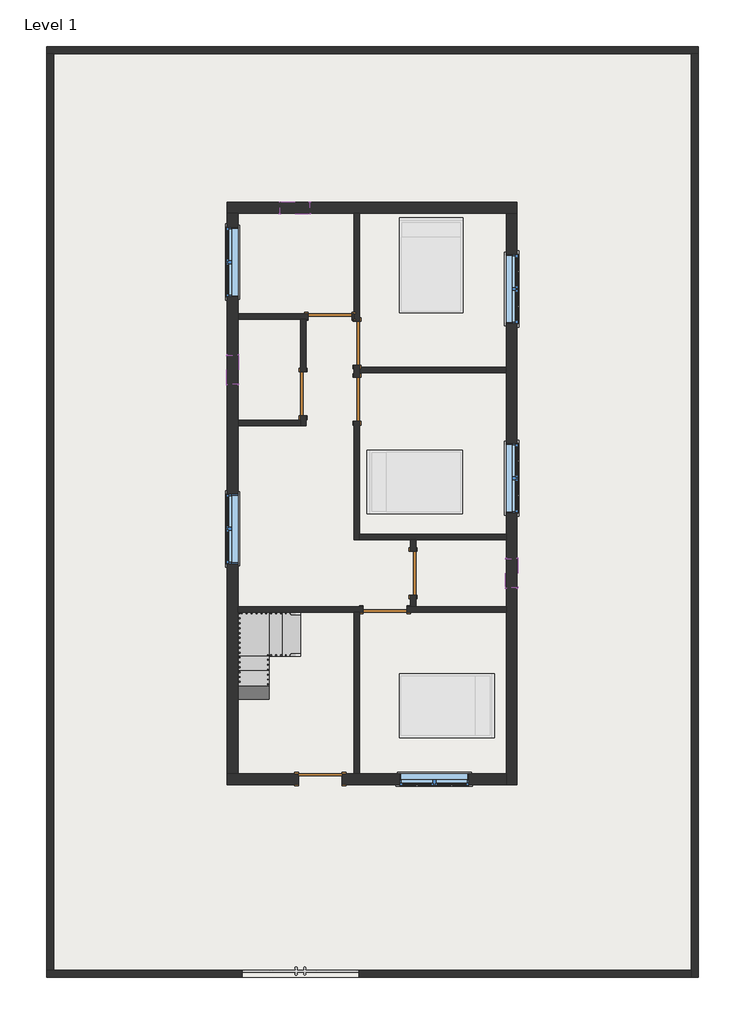
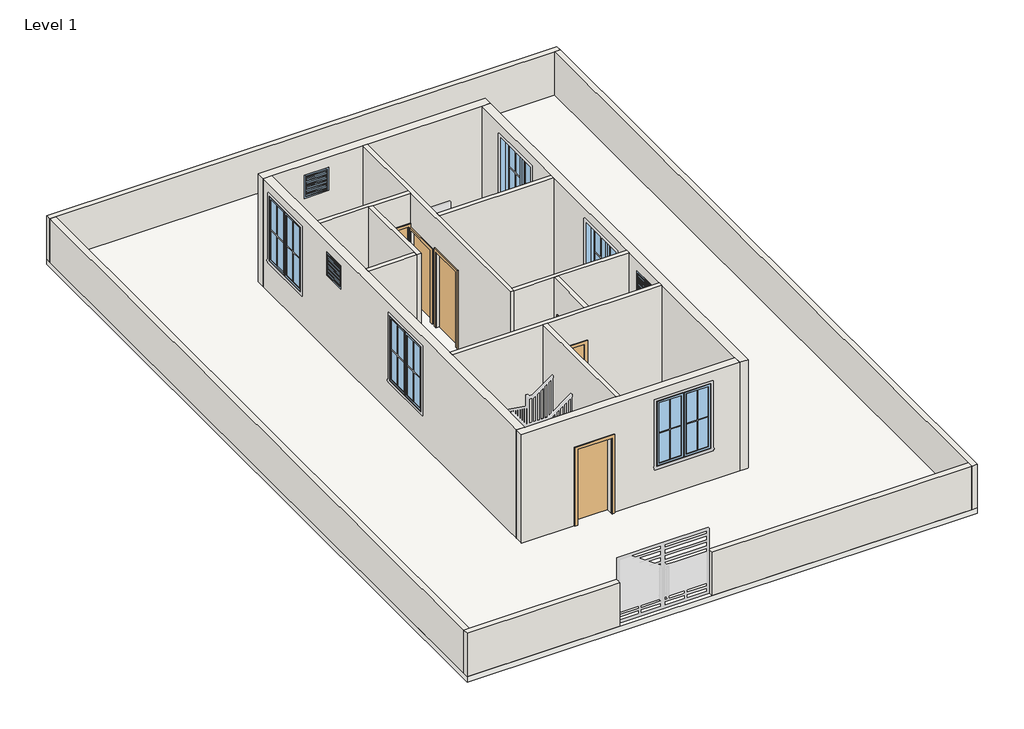
# One storey, part 1 of 2: 18 walls, 8 windows, 7 doors, 1 slab, 1 stair flight.
"""IFC4 building model written with IfcOpenShell, lengths in millimetres."""

from ifc_helpers import new_model, si_unit, frame, origin, origin_with_axes, place, context, project, spatial, polyline, outline, extrude, faceted_brep, transform, mapped, element, save
from components import door_5e62189b, door_17d80c48, door_e5f9f3c4, door_305aa2a5, door_0ca8825f, window_9ac97e1a, window_f2d8fef0

model = new_model("IFC4")

# Units and contexts
model_context = context("Model", 3, world=origin())
ifc_project = project(units=[si_unit("LENGTHUNIT", "METRE", prefix="MILLI")], contexts=[model_context])

# Site, building, storey
site = spatial("IfcSite", under=ifc_project)
building = spatial("IfcBuilding", under=site)
storey = spatial("IfcBuildingStorey", under=building, Name="Level 1", Elevation=0.0)

# Doors
placement = place(None, origin())
door_shape = door_5e62189b(model_context)
element("IfcDoor", 1, ObjectType="Single-Flush : 36\" x 80\"", at=placement, inside=storey, context=model_context, shape_type="MappedRepresentation", body=[
    mapped(door_shape, transform((-2690.3389285, 2204.6069249, 0.0), x_axis=(0.0, -1.0, 0.0), y_axis=(1.0, 0.0, 0.0), z_axis=(0.0, 0.0, 1.0))),
])
element("IfcDoor", 2, ObjectType="Single-Flush : 36\" x 80\"", at=placement, inside=storey, context=model_context, shape_type="MappedRepresentation", body=[
    mapped(door_shape, transform((-404.3389285, -1522.8430751, 0.0), x_axis=(0.0, 1.0, 0.0), y_axis=(-1.0, 0.0, 0.0), z_axis=(0.0, 0.0, 1.0))),
])
door_2_shape = door_17d80c48(model_context)
element("IfcDoor", 3, ObjectType="Single-Flush : 36\" x 80\"", at=placement, inside=storey, context=model_context, shape_type="MappedRepresentation", body=[
    mapped(door_2_shape, transform((-1572.7389285, 3258.7069249, 0.0), x_axis=(0.0, -1.0, 0.0), y_axis=(1.0, 0.0, 0.0), z_axis=(0.0, 0.0, 1.0))),
])
door_3_shape = door_e5f9f3c4(model_context)
element("IfcDoor", 4, ObjectType="Single-Flush : 36\" x 84\"", at=placement, inside=storey, context=model_context, shape_type="MappedRepresentation", body=[
    mapped(door_3_shape, transform((-2131.5389285, 3817.5069249, 0.0), x_axis=(1.0, 0.0, 0.0), y_axis=(0.0, 1.0, 0.0), z_axis=(0.0, 0.0, 1.0))),
])
element("IfcDoor", 5, ObjectType="Single-Flush : 36\" x 84\"", at=placement, inside=storey, context=model_context, shape_type="MappedRepresentation", body=[
    mapped(door_3_shape, transform((-988.5389285, -2278.4930751, 0.0), x_axis=(-1.0, 0.0, 0.0), y_axis=(0.0, -1.0, 0.0), z_axis=(0.0, 0.0, 1.0))),
])
door_4_shape = door_305aa2a5(model_context)
element("IfcDoor", 6, ObjectType="Single-Flush : 36\" x 84\"", at=placement, inside=storey, context=model_context, shape_type="MappedRepresentation", body=[
    mapped(door_4_shape, transform((-1572.7389285, 2090.3069249, 0.0), x_axis=(0.0, 1.0, 0.0), y_axis=(-1.0, 0.0, 0.0), z_axis=(0.0, 0.0, 1.0))),
])
door_5_shape = door_0ca8825f(model_context)
element("IfcDoor", 7, ObjectType="Single-Flush : 36\" x 84\"", at=placement, inside=storey, context=model_context, shape_type="MappedRepresentation", body=[
    mapped(door_5_shape, transform((-2334.7389285, -5802.7430751, 0.0), x_axis=(1.0, 0.0, 0.0), y_axis=(0.0, 1.0, 0.0), z_axis=(0.0, 0.0, 1.0))),
])

# Slab
element("IfcSlab", 8, ObjectType="FLOOR 6\"", at=placement, inside=storey, context=model_context, shape_type="SweptSolid", body=[
    extrude(outline(polyline([(5532.8162989, 9427.0671147), (5532.8162989, -9927.7328853), (-8030.7837011, -9927.7328853), (-8030.7837011, 9427.0671147), (5532.8162989, 9427.0671147)])), frame((0.0, 0.0, -152.4), z_axis=(0.0, 0.0, 1.0), x_axis=(1.0, 0.0, 0.0)), (0.0, 0.0, 1.0), 152.4),
])

# Stair flight
element("IfcStairFlight", 9, ObjectType="3/4\" Nosing", at=placement, inside=storey, context=model_context, shape_type="Brep", body=[
    faceted_brep([(-2747.4889285, -3250.0430751, 217.7142857), (-2747.4889285, -2335.6430751, 217.7142857), (-3128.4889285, -2335.6430751, 217.7142857), (-3128.4889285, -3250.0430751, 217.7142857), (-3128.4889285, -3250.0430751, 154.2142857), (-2753.0451785, -3250.0430751, 154.2142857), (-2753.0451785, -2335.6430751, 154.2142857), (-3128.4889285, -2335.6430751, 154.2142857)], [[[0, 1, 2, 3]], [[0, 3, 4, 5]], [[2, 1, 6, 7]], [[1, 0, 5, 6]], [[4, 7, 6, 5]], [[7, 4, 3, 2]]]),
    faceted_brep([(-3128.4889285, -3250.0430751, 435.4285714), (-3128.4889285, -2335.6430751, 435.4285714), (-3401.5389285, -2335.6430751, 435.4285714), (-3401.5389285, -3250.0430751, 435.4285714), (-3401.5389285, -3250.0430751, 371.9285714), (-3134.0451785, -3250.0430751, 371.9285714), (-3134.0451785, -2335.6430751, 371.9285714), (-3401.5389285, -2335.6430751, 371.9285714)], [[[0, 1, 2, 3]], [[0, 3, 4, 5]], [[2, 1, 6, 7]], [[1, 0, 5, 6]], [[4, 7, 6, 5]], [[7, 4, 3, 2]]]),
    faceted_brep([(-3401.5389285, -3269.0930751, 653.1428571), (-3401.5389285, -3250.0430751, 653.1428571), (-3401.5389285, -2335.6430751, 653.1428571), (-4042.8889285, -2335.6430751, 653.1428571), (-4042.8889285, -3269.0930751, 653.1428571), (-3401.5389285, -3269.0930751, 589.6428571), (-3401.5389285, -3250.0430751, 589.6428571), (-3407.0951785, -3250.0430751, 589.6428571), (-3407.0951785, -2335.6430751, 589.6428571), (-4042.8889285, -2335.6430751, 589.6428571), (-4042.8889285, -3269.0930751, 589.6428571), (-3401.5389285, -3250.0430751, 870.8571429), (-4042.8889285, -3250.0430751, 870.8571429), (-4042.8889285, -3289.4456691, 870.8571429), (-4042.8889285, -3573.8930751, 870.8571429), (-3401.5389285, -3573.8930751, 870.8571429), (-3401.5389285, -3289.4456691, 870.8571429), (-3401.5389285, -3573.8930751, 792.8571605), (-3401.5389285, -3289.4456691, 589.6428571), (-4042.8889285, -3289.4456691, 589.6428571), (-4042.8889285, -3573.8930751, 792.8571605), (-3401.5389285, -3554.8430751, 1088.5714286), (-4042.8889285, -3554.8430751, 1088.5714286), (-4042.8889285, -3878.6930751, 1088.5714286), (-3401.5389285, -3878.6930751, 1088.5714286), (-3401.5389285, -3878.6930751, 1010.6117202), (-4042.8889285, -3878.6930751, 1010.6117202), (-3401.5389285, -3859.6430751, 1306.2857143), (-4042.8889285, -3859.6430751, 1306.2857143), (-4042.8889285, -4183.4930751, 1306.2857143), (-3401.5389285, -4183.4930751, 1306.2857143), (-3401.5389285, -4183.4930751, 1228.36628), (-4042.8889285, -4183.4930751, 1228.36628), (-3401.5389285, -4164.4430751, 1524.0), (-4042.8889285, -4164.4430751, 1524.0), (-4042.8889285, -4488.2930751, 1524.0), (-3401.5389285, -4488.2930751, 1524.0), (-3401.5389285, -4488.2930751, 1446.1208397), (-4042.8889285, -4488.2930751, 1446.1208397), (-3401.5389285, -4792.8112092, 1741.7142857), (-3401.5389285, -4469.2430751, 1741.7142857), (-4042.8889285, -4469.2430751, 1741.7142857), (-4042.8889285, -4792.8112092, 1741.7142857), (-3401.5389285, -4773.7612092, 1959.4285714), (-3401.5389285, -5117.90743, 1959.4285714), (-3401.5389285, -5117.90743, 1895.9285714), (-4042.8889285, -4792.8112092, 1663.6740294), (-4042.8889285, -4773.7612092, 1959.4285714), (-4042.8889285, -5117.90743, 1959.4285714), (-4042.8889285, -5688.4430751, 1959.4285714), (-3401.5389285, -5688.4430751, 1959.4285714), (-4042.8889285, -5117.90743, 1895.9285714), (-4042.8889285, -5688.4430751, 1895.9285714), (-3401.5389285, -5688.4430751, 1895.9285714)], [[[0, 1, 2, 3, 4]], [[1, 0, 5, 6]], [[7, 1, 6]], [[3, 2, 8, 9]], [[4, 3, 9, 10]], [[11, 12, 13, 14, 15, 16]], [[0, 11, 16, 15, 17, 18, 5]], [[12, 4, 10, 19, 20, 14, 13]], [[21, 22, 23, 24]], [[21, 24, 25, 17, 15]], [[23, 22, 14, 20, 26]], [[27, 28, 29, 30]], [[27, 30, 31, 25, 24]], [[29, 28, 23, 26, 32]], [[33, 34, 35, 36]], [[33, 36, 37, 31, 30]], [[35, 34, 29, 32, 38]], [[39, 40, 41, 42]], [[39, 43, 44, 45, 37, 36, 40]], [[42, 41, 35, 38, 46]], [[43, 47, 48, 49, 50, 44]], [[47, 42, 46, 51, 52, 49, 48]], [[50, 49, 52, 53]], [[2, 1, 7, 8]], [[0, 4, 12, 11]], [[15, 14, 22, 21]], [[24, 23, 28, 27]], [[30, 29, 34, 33]], [[36, 35, 41, 40]], [[39, 42, 47, 43]], [[18, 19, 10, 9, 8, 7, 6, 5]], [[19, 18, 17, 25, 31, 37, 45, 51, 46, 38, 32, 26, 20]], [[45, 53, 52, 51]], [[53, 45, 44, 50]]]),
    faceted_brep([(-3401.5389285, -4773.7612092, 2177.1428571), (-3401.5389285, -5688.4430751, 2177.1428571), (-3128.4889285, -5688.4430751, 2177.1428571), (-3128.4889285, -4773.7612092, 2177.1428571), (-3395.9826785, -4773.7612092, 2113.6428571), (-3128.4889285, -4773.7612092, 2113.6428571), (-3395.9826785, -5688.4430751, 2113.6428571), (-3128.4889285, -5688.4430751, 2113.6428571)], [[[0, 1, 2, 3]], [[4, 0, 3, 5]], [[2, 1, 6, 7]], [[1, 0, 4, 6]], [[5, 7, 6, 4]], [[7, 5, 3, 2]]]),
    faceted_brep([(-3128.4889285, -4773.7612092, 2394.8571429), (-3128.4889285, -5688.4430751, 2394.8571429), (-2793.6303845, -5688.4430751, 2394.8571429), (-2793.6303845, -4773.7612092, 2394.8571429), (-2793.6303845, -4773.7612092, 2331.3571429), (-3122.9326785, -4773.7612092, 2331.3571429), (-3122.9326785, -5688.4430751, 2331.3571429), (-2793.6303845, -5688.4430751, 2331.3571429)], [[[0, 1, 2, 3]], [[0, 3, 4, 5]], [[2, 1, 6, 7]], [[3, 2, 7, 4]], [[1, 0, 5, 6]], [[6, 5, 4, 7]]]),
])

# Walls
element("IfcWall", 10, ObjectType="CMD 6\"", at=placement, inside=storey, context=model_context, shape_type="Brep", body=[
    faceted_brep([(-8030.7837011, 9274.6671147, 0.0), (-7878.3837011, 9274.6671147, 0.0), (5380.4162989, 9274.6671147, 0.0), (5532.8162989, 9274.6671147, 0.0), (5532.8162989, 9274.6671147, 1219.2), (5380.4162989, 9274.6671147, 1219.2), (-7878.3837011, 9274.6671147, 1219.2), (-8030.7837011, 9274.6671147, 1219.2), (-8030.7837011, 9427.0671147, 0.0), (-8030.7837011, 9427.0671147, 1219.2), (5532.8162989, 9427.0671147, 1219.2), (5532.8162989, 9427.0671147, 0.0)], [[[0, 1, 2, 3, 4, 5, 6, 7]], [[8, 9, 10, 11]], [[3, 2, 1, 0, 8, 11]], [[7, 6, 5, 4, 10, 9]], [[4, 3, 11, 10]], [[0, 7, 9, 8]]]),
])
element("IfcWall", 11, ObjectType="CMD 6\"", at=placement, inside=storey, context=model_context, shape_type="Brep", body=[
    faceted_brep([(5380.4162989, 9274.6671147, 0.0), (5380.4162989, -9775.3328853, 0.0), (5380.4162989, -9927.7328853, 0.0), (5380.4162989, -9927.7328853, 1219.2), (5380.4162989, -9775.3328853, 1219.2), (5380.4162989, 9274.6671147, 1219.2), (5532.8162989, 9274.6671147, 0.0), (5532.8162989, 9274.6671147, 1219.2), (5532.8162989, -9927.7328853, 1219.2), (5532.8162989, -9927.7328853, 0.0)], [[[0, 1, 2, 3, 4, 5]], [[6, 7, 8, 9]], [[2, 1, 0, 6, 9]], [[5, 4, 3, 8, 7]], [[0, 5, 7, 6]], [[3, 2, 9, 8]]]),
])
element("IfcWall", 12, ObjectType="CMD 6\"", at=placement, inside=storey, context=model_context, shape_type="SweptSolid", body=[
    extrude(outline(polyline([(-1528.2889285, -9775.3328853), (5380.4162989, -9775.3328853), (5380.4162989, -9927.7328853), (-1528.2889285, -9927.7328853), (-1528.2889285, -9775.3328853)])), origin_with_axes(), (0.0, 0.0, 1.0), 1219.2),
])
element("IfcWall", 13, ObjectType="CMD 6\"", at=placement, inside=storey, context=model_context, shape_type="SweptSolid", body=[
    extrude(outline(polyline([(-7878.3837011, 9274.6671147), (-7878.3837011, -9775.3328853), (-8030.7837011, -9775.3328853), (-8030.7837011, 9274.6671147), (-7878.3837011, 9274.6671147)])), origin_with_axes(), (0.0, 0.0, 1.0), 1219.2),
])
element("IfcWall", 14, ObjectType="CMD 6\"", at=placement, inside=storey, context=model_context, shape_type="Brep", body=[
    faceted_brep([(-3966.6889285, -9775.3328853, 0.0), (-7878.3837011, -9775.3328853, 0.0), (-8030.7837011, -9775.3328853, 0.0), (-8030.7837011, -9775.3328853, 1219.2), (-7878.3837011, -9775.3328853, 1219.2), (-3966.6889285, -9775.3328853, 1219.2), (-3966.6889285, -9927.7328853, 0.0), (-3966.6889285, -9927.7328853, 1219.2), (-8030.7837011, -9927.7328853, 1219.2), (-8030.7837011, -9927.7328853, 0.0)], [[[0, 1, 2, 3, 4, 5]], [[6, 7, 8, 9]], [[2, 1, 0, 6, 9]], [[5, 4, 3, 8, 7]], [[0, 5, 7, 6]], [[3, 2, 9, 8]]]),
])
element("IfcWall", 15, ObjectType="WALL 4.5\"", at=placement, inside=storey, context=model_context, shape_type="Brep", body=[
    faceted_brep([(-1629.8889285, 2801.5069249, 2032.0), (-1629.8889285, 2801.5069249, 0.0), (-1629.8889285, 2547.5069249, 0.0), (-1629.8889285, 2547.5069249, 2133.6), (-1629.8889285, 1633.1069249, 2133.6), (-1629.8889285, 1633.1069249, 0.0), (-1629.8889285, -824.3430751, 0.0), (-1629.8889285, -824.3430751, 3048.0), (-1629.8889285, 3760.3569249, 3048.0), (-1629.8889285, 3874.6569249, 3048.0), (-1629.8889285, 5957.4569249, 3048.0), (-1629.8889285, 5957.4569249, 0.0), (-1629.8889285, 3874.6569249, 0.0), (-1629.8889285, 3760.3569249, 0.0), (-1629.8889285, 3715.9069249, 0.0), (-1629.8889285, 3715.9069249, 2032.0), (-1515.5889285, 2547.5069249, 0.0), (-1515.5889285, 2642.7569249, 0.0), (-1515.5889285, 2757.0569249, 0.0), (-1515.5889285, 2801.5069249, 0.0), (-1515.5889285, 2801.5069249, 2032.0), (-1515.5889285, 3715.9069249, 2032.0), (-1515.5889285, 3715.9069249, 0.0), (-1515.5889285, 5957.4569249, 0.0), (-1515.5889285, 5957.4569249, 3048.0), (-1515.5889285, 2757.0569249, 3048.0), (-1515.5889285, 2642.7569249, 3048.0), (-1515.5889285, -710.0430751, 3048.0), (-1515.5889285, -824.3430751, 3048.0), (-1515.5889285, -824.3430751, 0.0), (-1515.5889285, -710.0430751, 0.0), (-1515.5889285, 1633.1069249, 0.0), (-1515.5889285, 1633.1069249, 2133.6), (-1515.5889285, 2547.5069249, 2133.6)], [[[0, 1, 2, 3, 4, 5, 6, 7, 8, 9, 10, 11, 12, 13, 14, 15]], [[16, 17, 18, 19, 20, 21, 22, 23, 24, 25, 26, 27, 28, 29, 30, 31, 32, 33]], [[31, 30, 29, 6, 5]], [[2, 1, 19, 18, 17, 16]], [[14, 13, 12, 11, 23, 22]], [[7, 6, 29, 28]], [[11, 10, 24, 23]], [[3, 2, 16, 33]], [[4, 3, 33, 32]], [[5, 4, 32, 31]], [[20, 19, 1, 0]], [[21, 20, 0, 15]], [[22, 21, 15, 14]], [[10, 9, 8, 7, 28, 27, 26, 25, 24]]]),
])
element("IfcWall", 16, ObjectType="WALL 4.5\"", at=placement, inside=storey, context=model_context, shape_type="Brep", body=[
    faceted_brep([(1532.4110715, -710.0430751, 0.0), (-1515.5889285, -710.0430751, 0.0), (-1515.5889285, -710.0430751, 3048.0), (1532.4110715, -710.0430751, 3048.0), (1532.4110715, -824.3430751, 0.0), (1532.4110715, -824.3430751, 3048.0), (-347.1889285, -824.3430751, 3048.0), (-461.4889285, -824.3430751, 3048.0), (-1515.5889285, -824.3430751, 3048.0), (-1515.5889285, -824.3430751, 0.0), (-461.4889285, -824.3430751, 0.0), (-347.1889285, -824.3430751, 0.0)], [[[0, 1, 2, 3]], [[4, 5, 6, 7, 8, 9, 10, 11]], [[1, 0, 4, 11, 10, 9]], [[0, 3, 5, 4]], [[2, 1, 9, 8]], [[3, 2, 8, 7, 6, 5]]]),
])
element("IfcWall", 17, ObjectType="WALL 4.5\"", at=placement, inside=storey, context=model_context, shape_type="SweptSolid", body=[
    extrude(outline(polyline([(-1515.5889285, 2757.0569249), (1532.4110715, 2757.0569249), (1532.4110715, 2642.7569249), (-1515.5889285, 2642.7569249), (-1515.5889285, 2757.0569249)])), origin_with_axes(), (0.0, 0.0, 1.0), 3048.0),
])
element("IfcWall", 18, ObjectType="WALL 4.5\"", at=placement, inside=storey, context=model_context, shape_type="Brep", body=[
    faceted_brep([(-1674.3389285, 3760.3569249, 2133.6), (-1674.3389285, 3760.3569249, 0.0), (-1629.8889285, 3760.3569249, 0.0), (-1629.8889285, 3760.3569249, 3048.0), (-2633.1889285, 3760.3569249, 3048.0), (-2747.4889285, 3760.3569249, 3048.0), (-4042.8889285, 3760.3569249, 3048.0), (-4042.8889285, 3760.3569249, 0.0), (-2747.4889285, 3760.3569249, 0.0), (-2633.1889285, 3760.3569249, 0.0), (-2588.7389285, 3760.3569249, 0.0), (-2588.7389285, 3760.3569249, 2133.6), (-1629.8889285, 3874.6569249, 0.0), (-1674.3389285, 3874.6569249, 0.0), (-1674.3389285, 3874.6569249, 2133.6), (-2588.7389285, 3874.6569249, 2133.6), (-2588.7389285, 3874.6569249, 0.0), (-4042.8889285, 3874.6569249, 0.0), (-4042.8889285, 3874.6569249, 3048.0), (-1629.8889285, 3874.6569249, 3048.0)], [[[0, 1, 2, 3, 4, 5, 6, 7, 8, 9, 10, 11]], [[12, 13, 14, 15, 16, 17, 18, 19]], [[2, 1, 13, 12]], [[10, 9, 8, 7, 17, 16]], [[7, 6, 18, 17]], [[3, 2, 12, 19]], [[14, 13, 1, 0]], [[15, 14, 0, 11]], [[16, 15, 11, 10]], [[6, 5, 4, 3, 19, 18]]]),
])
element("IfcWall", 19, ObjectType="WALL 4.5\"", at=placement, inside=storey, context=model_context, shape_type="Brep", body=[
    faceted_brep([(-2747.4889285, 1747.4069249, 2032.0), (-2747.4889285, 1747.4069249, 0.0), (-2747.4889285, 1652.1569249, 0.0), (-2747.4889285, 1537.8569249, 0.0), (-2747.4889285, 1537.8569249, 3048.0), (-2747.4889285, 1652.1569249, 3048.0), (-2747.4889285, 3760.3569249, 3048.0), (-2747.4889285, 3760.3569249, 0.0), (-2747.4889285, 2661.8069249, 0.0), (-2747.4889285, 2661.8069249, 2032.0), (-2633.1889285, 1537.8569249, 0.0), (-2633.1889285, 1747.4069249, 0.0), (-2633.1889285, 1747.4069249, 2032.0), (-2633.1889285, 2661.8069249, 2032.0), (-2633.1889285, 2661.8069249, 0.0), (-2633.1889285, 3760.3569249, 0.0), (-2633.1889285, 3760.3569249, 3048.0), (-2633.1889285, 1537.8569249, 3048.0)], [[[0, 1, 2, 3, 4, 5, 6, 7, 8, 9]], [[10, 11, 12, 13, 14, 15, 16, 17]], [[8, 7, 15, 14]], [[3, 2, 1, 11, 10]], [[7, 6, 16, 15]], [[4, 3, 10, 17]], [[12, 11, 1, 0]], [[13, 12, 0, 9]], [[14, 13, 9, 8]], [[6, 5, 4, 17, 16]]]),
])
element("IfcWall", 20, ObjectType="WALL 4.5\"", at=placement, inside=storey, context=model_context, shape_type="SweptSolid", body=[
    extrude(outline(polyline([(-4042.8889285, 1652.1569249), (-2747.4889285, 1652.1569249), (-2747.4889285, 1537.8569249), (-4042.8889285, 1537.8569249), (-4042.8889285, 1652.1569249)])), origin_with_axes(), (0.0, 0.0, 1.0), 3048.0),
])
element("IfcWall", 21, ObjectType="WALL 4.5\"", at=placement, inside=storey, context=model_context, shape_type="Brep", body=[
    faceted_brep([(-4042.8889285, -2335.6430751, 0.0), (-1629.8889285, -2335.6430751, 0.0), (-1515.5889285, -2335.6430751, 0.0), (-1445.7389285, -2335.6430751, 0.0), (-1445.7389285, -2335.6430751, 2133.6), (-531.3389285, -2335.6430751, 2133.6), (-531.3389285, -2335.6430751, 0.0), (1532.4110715, -2335.6430751, 0.0), (1532.4110715, -2335.6430751, 3048.0), (-1515.5889285, -2335.6430751, 3048.0), (-1629.8889285, -2335.6430751, 3048.0), (-4042.8889285, -2335.6430751, 3048.0), (-1445.7389285, -2221.3430751, 2133.6), (-1445.7389285, -2221.3430751, 0.0), (-4042.8889285, -2221.3430751, 0.0), (-4042.8889285, -2221.3430751, 3048.0), (-461.4889285, -2221.3430751, 3048.0), (-347.1889285, -2221.3430751, 3048.0), (1532.4110715, -2221.3430751, 3048.0), (1532.4110715, -2221.3430751, 0.0), (-347.1889285, -2221.3430751, 0.0), (-461.4889285, -2221.3430751, 0.0), (-531.3389285, -2221.3430751, 0.0), (-531.3389285, -2221.3430751, 2133.6)], [[[0, 1, 2, 3, 4, 5, 6, 7, 8, 9, 10, 11]], [[12, 13, 14, 15, 16, 17, 18, 19, 20, 21, 22, 23]], [[14, 13, 3, 2, 1, 0]], [[22, 21, 20, 19, 7, 6]], [[8, 7, 19, 18]], [[0, 11, 15, 14]], [[4, 3, 13, 12]], [[5, 4, 12, 23]], [[6, 5, 23, 22]], [[11, 10, 9, 8, 18, 17, 16, 15]]]),
])
element("IfcWall", 22, ObjectType="WALL 4.5\"", at=placement, inside=storey, context=model_context, shape_type="SweptSolid", body=[
    extrude(outline(polyline([(-824.3430751, 0.0), (-1065.6430751, 0.0), (-1065.6430751, 2032.0), (-1980.0430751, 2032.0), (-1980.0430751, 0.0), (-2221.3430751, 0.0), (-2221.3430751, 3048.0), (-824.3430751, 3048.0), (-824.3430751, 0.0)])), frame((-461.4889285, 0.0, 0.0), z_axis=(1.0, 0.0, 0.0), x_axis=(0.0, 1.0, 0.0)), (0.0, 0.0, 1.0), 114.3),
])
element("IfcWall", 23, ObjectType="WALL 4.5\"", at=placement, inside=storey, context=model_context, shape_type="SweptSolid", body=[
    extrude(outline(polyline([(-1629.8889285, -5688.4430751), (-1629.8889285, -2335.6430751), (-1515.5889285, -2335.6430751), (-1515.5889285, -5688.4430751), (-1629.8889285, -5688.4430751)])), origin_with_axes(), (0.0, 0.0, 1.0), 3048.0),
])
element("IfcWall", 24, ObjectType="WALL 9\"", at=placement, inside=storey, context=model_context, shape_type="Brep", body=[
    faceted_brep([(-4271.4889285, 5957.4569249, 0.0), (-4042.8889285, 5957.4569249, 0.0), (-1629.8889285, 5957.4569249, 0.0), (-1515.5889285, 5957.4569249, 0.0), (1532.4110715, 5957.4569249, 0.0), (1761.0110715, 5957.4569249, 0.0), (1761.0110715, 5957.4569249, 3048.0), (1532.4110715, 5957.4569249, 3048.0), (-1515.5889285, 5957.4569249, 3048.0), (-1629.8889285, 5957.4569249, 3048.0), (-4042.8889285, 5957.4569249, 3048.0), (-4271.4889285, 5957.4569249, 3048.0), (-2560.1639285, 5957.4569249, 2743.2), (-2560.1639285, 5957.4569249, 2133.6), (-3169.7639285, 5957.4569249, 2133.6), (-3169.7639285, 5957.4569249, 2743.2), (-4271.4889285, 6186.0569249, 0.0), (-4271.4889285, 6186.0569249, 3048.0), (1761.0110715, 6186.0569249, 3048.0), (1761.0110715, 6186.0569249, 0.0), (-2560.1639285, 6186.0569249, 2743.2), (-3169.7639285, 6186.0569249, 2743.2), (-3169.7639285, 6186.0569249, 2133.6), (-2560.1639285, 6186.0569249, 2133.6)], [[[0, 1, 2, 3, 4, 5, 6, 7, 8, 9, 10, 11], [12, 13, 14, 15]], [[16, 17, 18, 19], [20, 21, 22, 23]], [[5, 4, 3, 2, 1, 0, 16, 19]], [[6, 5, 19, 18]], [[0, 11, 17, 16]], [[13, 12, 20, 23]], [[14, 13, 23, 22]], [[15, 14, 22, 21]], [[12, 15, 21, 20]], [[11, 10, 9, 8, 7, 6, 18, 17]]]),
])
element("IfcWall", 25, ObjectType="WALL 9\"", at=placement, inside=storey, context=model_context, shape_type="Brep", body=[
    faceted_brep([(1532.4110715, 5957.4569249, 0.0), (1532.4110715, 2757.0569249, 0.0), (1532.4110715, 2642.7569249, 0.0), (1532.4110715, -710.0430751, 0.0), (1532.4110715, -824.3430751, 0.0), (1532.4110715, -2221.3430751, 0.0), (1532.4110715, -2335.6430751, 0.0), (1532.4110715, -5688.4430751, 0.0), (1532.4110715, -5917.0430751, 0.0), (1532.4110715, -5917.0430751, 3048.0), (1532.4110715, -5688.4430751, 3048.0), (1532.4110715, -2335.6430751, 3048.0), (1532.4110715, -2221.3430751, 3048.0), (1532.4110715, -824.3430751, 3048.0), (1532.4110715, -710.0430751, 3048.0), (1532.4110715, 2642.7569249, 3048.0), (1532.4110715, 2757.0569249, 3048.0), (1532.4110715, 5957.4569249, 3048.0), (1532.4110715, 3661.9319249, 2743.2), (1532.4110715, 3661.9319249, 914.4), (1532.4110715, 5109.7319249, 914.4), (1532.4110715, 5109.7319249, 2743.2), (1532.4110715, -271.8930751, 2743.2), (1532.4110715, -271.8930751, 914.4), (1532.4110715, 1175.9069249, 914.4), (1532.4110715, 1175.9069249, 2743.2), (1532.4110715, -1827.6430751, 2743.2), (1532.4110715, -1827.6430751, 2133.6), (1532.4110715, -1218.0430751, 2133.6), (1532.4110715, -1218.0430751, 2743.2), (1761.0110715, 5957.4569249, 0.0), (1761.0110715, 5957.4569249, 3048.0), (1761.0110715, -5917.0430751, 3048.0), (1761.0110715, -5917.0430751, 0.0), (1761.0110715, 3661.9319249, 2743.2), (1761.0110715, 5109.7319249, 2743.2), (1761.0110715, 5109.7319249, 914.4), (1761.0110715, 3661.9319249, 914.4), (1761.0110715, -271.8930751, 2743.2), (1761.0110715, 1175.9069249, 2743.2), (1761.0110715, 1175.9069249, 914.4), (1761.0110715, -271.8930751, 914.4), (1761.0110715, -1827.6430751, 2743.2), (1761.0110715, -1218.0430751, 2743.2), (1761.0110715, -1218.0430751, 2133.6), (1761.0110715, -1827.6430751, 2133.6)], [[[0, 1, 2, 3, 4, 5, 6, 7, 8, 9, 10, 11, 12, 13, 14, 15, 16, 17], [18, 19, 20, 21], [22, 23, 24, 25], [26, 27, 28, 29]], [[30, 31, 32, 33], [34, 35, 36, 37], [38, 39, 40, 41], [42, 43, 44, 45]], [[8, 7, 6, 5, 4, 3, 2, 1, 0, 30, 33]], [[0, 17, 31, 30]], [[9, 8, 33, 32]], [[19, 18, 34, 37]], [[20, 19, 37, 36]], [[21, 20, 36, 35]], [[18, 21, 35, 34]], [[23, 22, 38, 41]], [[24, 23, 41, 40]], [[25, 24, 40, 39]], [[22, 25, 39, 38]], [[27, 26, 42, 45]], [[28, 27, 45, 44]], [[29, 28, 44, 43]], [[26, 29, 43, 42]], [[17, 16, 15, 14, 13, 12, 11, 10, 9, 32, 31]]]),
])
element("IfcWall", 26, ObjectType="WALL 9\"", at=placement, inside=storey, context=model_context, shape_type="Brep", body=[
    faceted_brep([(1532.4110715, -5688.4430751, 0.0), (-1515.5889285, -5688.4430751, 0.0), (-1629.8889285, -5688.4430751, 0.0), (-1877.5389285, -5688.4430751, 0.0), (-1877.5389285, -5688.4430751, 2133.6), (-2791.9389285, -5688.4430751, 2133.6), (-2791.9389285, -5688.4430751, 0.0), (-4042.8889285, -5688.4430751, 0.0), (-4271.4889285, -5688.4430751, 0.0), (-4271.4889285, -5688.4430751, 3048.0), (-4042.8889285, -5688.4430751, 3048.0), (-1629.8889285, -5688.4430751, 3048.0), (-1515.5889285, -5688.4430751, 3048.0), (1532.4110715, -5688.4430751, 3048.0), (-686.9139285, -5688.4430751, 2743.2), (-686.9139285, -5688.4430751, 914.4), (760.8860715, -5688.4430751, 914.4), (760.8860715, -5688.4430751, 2743.2), (-1877.5389285, -5917.0430751, 2133.6), (-1877.5389285, -5917.0430751, 0.0), (1532.4110715, -5917.0430751, 0.0), (1532.4110715, -5917.0430751, 3048.0), (-4271.4889285, -5917.0430751, 3048.0), (-4271.4889285, -5917.0430751, 0.0), (-2791.9389285, -5917.0430751, 0.0), (-2791.9389285, -5917.0430751, 2133.6), (-686.9139285, -5917.0430751, 2743.2), (760.8860715, -5917.0430751, 2743.2), (760.8860715, -5917.0430751, 914.4), (-686.9139285, -5917.0430751, 914.4)], [[[0, 1, 2, 3, 4, 5, 6, 7, 8, 9, 10, 11, 12, 13], [14, 15, 16, 17]], [[18, 19, 20, 21, 22, 23, 24, 25], [26, 27, 28, 29]], [[24, 23, 8, 7, 6]], [[20, 19, 3, 2, 1, 0]], [[0, 13, 21, 20]], [[9, 8, 23, 22]], [[15, 14, 26, 29]], [[16, 15, 29, 28]], [[17, 16, 28, 27]], [[14, 17, 27, 26]], [[4, 3, 19, 18]], [[5, 4, 18, 25]], [[6, 5, 25, 24]], [[13, 12, 11, 10, 9, 22, 21]]]),
])
element("IfcWall", 27, ObjectType="WALL 9\"", at=placement, inside=storey, context=model_context, shape_type="Brep", body=[
    faceted_brep([(-4042.8889285, -5688.4430751, 0.0), (-4042.8889285, -2335.6430751, 0.0), (-4042.8889285, -2221.3430751, 0.0), (-4042.8889285, 1537.8569249, 0.0), (-4042.8889285, 1652.1569249, 0.0), (-4042.8889285, 3760.3569249, 0.0), (-4042.8889285, 3874.6569249, 0.0), (-4042.8889285, 5957.4569249, 0.0), (-4042.8889285, 5957.4569249, 3048.0), (-4042.8889285, 3874.6569249, 3048.0), (-4042.8889285, 3760.3569249, 3048.0), (-4042.8889285, 1652.1569249, 3048.0), (-4042.8889285, 1537.8569249, 3048.0), (-4042.8889285, -2221.3430751, 3048.0), (-4042.8889285, -2335.6430751, 3048.0), (-4042.8889285, -5688.4430751, 3048.0), (-4042.8889285, 5668.5319249, 2743.2), (-4042.8889285, 5668.5319249, 914.4), (-4042.8889285, 4220.7319249, 914.4), (-4042.8889285, 4220.7319249, 2743.2), (-4042.8889285, 121.8069249, 2743.2), (-4042.8889285, 121.8069249, 914.4), (-4042.8889285, -1325.9930751, 914.4), (-4042.8889285, -1325.9930751, 2743.2), (-4042.8889285, 2401.4569249, 2743.2), (-4042.8889285, 3011.0569249, 2743.2), (-4042.8889285, 3011.0569249, 2133.6), (-4042.8889285, 2401.4569249, 2133.6), (-4271.4889285, -5688.4430751, 0.0), (-4271.4889285, -5688.4430751, 3048.0), (-4271.4889285, 5957.4569249, 3048.0), (-4271.4889285, 5957.4569249, 0.0), (-4271.4889285, 5668.5319249, 2743.2), (-4271.4889285, 4220.7319249, 2743.2), (-4271.4889285, 4220.7319249, 914.4), (-4271.4889285, 5668.5319249, 914.4), (-4271.4889285, 121.8069249, 2743.2), (-4271.4889285, -1325.9930751, 2743.2), (-4271.4889285, -1325.9930751, 914.4), (-4271.4889285, 121.8069249, 914.4), (-4271.4889285, 2401.4569249, 2743.2), (-4271.4889285, 2401.4569249, 2133.6), (-4271.4889285, 3011.0569249, 2133.6), (-4271.4889285, 3011.0569249, 2743.2)], [[[0, 1, 2, 3, 4, 5, 6, 7, 8, 9, 10, 11, 12, 13, 14, 15], [16, 17, 18, 19], [20, 21, 22, 23], [24, 25, 26, 27]], [[28, 29, 30, 31], [32, 33, 34, 35], [36, 37, 38, 39], [40, 41, 42, 43]], [[7, 6, 5, 4, 3, 2, 1, 0, 28, 31]], [[0, 15, 29, 28]], [[8, 7, 31, 30]], [[17, 16, 32, 35]], [[18, 17, 35, 34]], [[19, 18, 34, 33]], [[16, 19, 33, 32]], [[21, 20, 36, 39]], [[22, 21, 39, 38]], [[23, 22, 38, 37]], [[20, 23, 37, 36]], [[41, 40, 24, 27]], [[42, 41, 27, 26]], [[43, 42, 26, 25]], [[40, 43, 25, 24]], [[15, 14, 13, 12, 11, 10, 9, 8, 30, 29]]]),
])

# Windows
window_shape = window_9ac97e1a(model_context)
element("IfcWindow", 28, ObjectType="Window-Casement-Double : 57\" x 72\"", at=placement, inside=storey, context=model_context, shape_type="MappedRepresentation", body=[
    mapped(window_shape, transform((-4157.1889285, 4944.6319249, 0.0), x_axis=(0.0, 1.0, 0.0), y_axis=(-1.0, 0.0, 0.0), z_axis=(0.0, 0.0, 1.0))),
])
element("IfcWindow", 29, ObjectType="Window-Casement-Double : 57\" x 72\"", at=placement, inside=storey, context=model_context, shape_type="MappedRepresentation", body=[
    mapped(window_shape, transform((1646.7110715, 4385.8319249, 0.0), x_axis=(0.0, -1.0, 0.0), y_axis=(1.0, 0.0, 0.0), z_axis=(0.0, 0.0, 1.0))),
])
element("IfcWindow", 30, ObjectType="Window-Casement-Double : 57\" x 72\"", at=placement, inside=storey, context=model_context, shape_type="MappedRepresentation", body=[
    mapped(window_shape, transform((-4157.1889285, -602.0930751, 0.0), x_axis=(0.0, 1.0, 0.0), y_axis=(-1.0, 0.0, 0.0), z_axis=(0.0, 0.0, 1.0))),
])
element("IfcWindow", 31, ObjectType="Window-Casement-Double : 57\" x 72\"", at=placement, inside=storey, context=model_context, shape_type="MappedRepresentation", body=[
    mapped(window_shape, transform((1646.7110715, 452.0069249, 0.0), x_axis=(0.0, -1.0, 0.0), y_axis=(1.0, 0.0, 0.0), z_axis=(0.0, 0.0, 1.0))),
])
element("IfcWindow", 32, ObjectType="Window-Casement-Double : 57\" x 72\"", at=placement, inside=storey, context=model_context, shape_type="MappedRepresentation", body=[
    mapped(window_shape, transform((36.9860715, -5802.7430751, 0.0), x_axis=(-1.0, 0.0, 0.0), y_axis=(0.0, -1.0, 0.0), z_axis=(0.0, 0.0, 1.0))),
])
window_2_shape = window_f2d8fef0(model_context)
element("IfcWindow", 33, ObjectType="Window-Louvers : 24\" x 24\"", at=placement, inside=storey, context=model_context, shape_type="MappedRepresentation", body=[
    mapped(window_2_shape, transform((-2864.9639285, 6065.4069249, 1219.2), x_axis=(-1.0, 0.0, 0.0), y_axis=(0.0, -1.0, 0.0), z_axis=(0.0, 0.0, 1.0))),
])
element("IfcWindow", 34, ObjectType="Window-Louvers : 24\" x 24\"", at=placement, inside=storey, context=model_context, shape_type="MappedRepresentation", body=[
    mapped(window_2_shape, transform((-4163.5389285, 2706.2569249, 1219.2), x_axis=(0.0, 1.0, 0.0), y_axis=(-1.0, 0.0, 0.0), z_axis=(0.0, 0.0, 1.0))),
])
element("IfcWindow", 35, ObjectType="Window-Louvers : 24\" x 24\"", at=placement, inside=storey, context=model_context, shape_type="MappedRepresentation", body=[
    mapped(window_2_shape, transform((1640.3610715, -1522.8430751, 1219.2), x_axis=(0.0, 1.0, 0.0), y_axis=(-1.0, 0.0, 0.0), z_axis=(0.0, 0.0, 1.0))),
])

save(model, "model.ifc")

# Revit data of these elements
# Type "Single-Flush : 36\" x 80\""
#   Type Mark = "6"
#   Construction Type Id = "MDOOR"
#   Assembly Code = "C1020"
#   Analytic Construction = "Metal"
#   Thickness = 0' - 2"
#   Heat Transfer Coefficient (U) = 0.651978 BTU/(h·ft²·°F)
#   Height = 6' - 8"
#   Trim Projection Ext = 0' - 1"
#   Trim Projection Int = 0' - 1"
#   Trim Width = 0' - 3"
#   Width = 3' - 0"
#   Define Thermal Properties by = 1
#   Define Thermal Properties by = 1
#   Door Material = Door - Panel
#   Frame Material = Door - Frame
#   Visual Light Transmittance = 0
#   Solar Heat Gain Coefficient = 0
#   Function = (empty or 0)
#   Wall Closure = (empty or 0)
# Type "Single-Flush : 36\" x 84\""
#   Type Mark = "1"
#   Construction Type Id = "MDOOR"
#   Assembly Code = "C1020"
#   Analytic Construction = "Metal"
#   Thickness = 0' - 2"
#   Heat Transfer Coefficient (U) = 0.651978 BTU/(h·ft²·°F)
#   Height = 7' - 0"
#   Trim Projection Ext = 0' - 1"
#   Trim Projection Int = 0' - 1"
#   Trim Width = 0' - 3"
#   Width = 3' - 0"
#   Define Thermal Properties by = 1
#   Define Thermal Properties by = 1
#   Door Material = Door - Panel
#   Frame Material = Door - Frame
#   Visual Light Transmittance = 0
#   Solar Heat Gain Coefficient = 0
#   Function = (empty or 0)
#   Wall Closure = (empty or 0)
# Type "FLOOR 6\""
#   Assembly Code = "B1010"
#   Function = 0
#   Layers, outside or top first: 0' - 6" no material (function 1)
# Type "CMD 6\""
#   Assembly Code = "B2010"
#   Layers, outside or top first: 0' - 6" no material (function 1)
# Type "WALL 4.5\""
#   Assembly Code = "B2010"
#   Layers, outside or top first: 0' - 4 1/2" no material (function 1)
# Type "WALL 9\""
#   Assembly Code = "B2010"
#   Layers, outside or top first: 0' - 9" no material (function 1)
# Type "Window-Casement-Double : 57\" x 72\""
#   Type Mark = "17"
#   Fire Rating = "0.5h"
#   Assembly Code = "B2020100"
#   Analytic Construction = "Double glazing - domestic"
#   Frame Extension [instance default] = 0' - 0 1/4"
#   Window Inset [instance default] = 0' - 0"
#   Wall Thickness [instance default] = 0' - 6"
#   Interior Wall Closure [instance default] = 0' - 2 1/4"
#   Half Width = 2' - 4 1/2"
#   Visual Light Transmittance = 0.81
#   Thermal Resistance (R) = 1.8146 (h·ft²·°F)/BTU
#   Solar Heat Gain Coefficient = 0.76
#   Rough Width = 4' - 9 1/2"
#   Rough Height = 6' - 0 1/2"
#   Height = 6' - 0"
#   Heat Transfer Coefficient (U) = 0.5511 BTU/(h·ft²·°F)
#   Exterior Wall Closure [instance default] = 0' - 1 1/4"
#   Extension Jamb [instance default] = 0' - 2 1/4"
#   Default Sill Height = 3' - 0"
#   Width = 4' - 9"
#   Define Thermal Properties by = 0
#   Muntin Visibility = yes
#   Interior Trim Visibility [instance default] = yes
#   Exterior Trim Visibility [instance default] = yes
#   Extension Jamb Visibility [instance default] = yes
#   Interior Trim Material = Wood - Stained
#   Muntin Pattern = Muntin Pattern_2x2 : Muntin Pattern_2x2
#   Interior Trim = Trim-Window-Interior-Flat : Picture Frame
#   Interior Frame Material = Wood - Stained
#   Glass Panel Material = Glass
#   Exterior Trim Material = Clad - White
#   Exterior Trim = Trim-Window-Exterior-Flat : with Sill
#   Exterior Frame Material = Clad - White
#   Wall Closure = (empty or 0)
# Type "Window-Louvers : 24\" x 24\""
#   Type Mark = "18"
#   Construction Type Id = "GSP4R"
#   Assembly Code = "B20"
#   Analytic Construction = "1/8 in Pilkington single glazing"
#   Visual Light Transmittance = 0.9
#   Thermal Resistance (R) = 1.53941 (h·ft²·°F)/BTU
#   Solar Heat Gain Coefficient = 0.78
#   Max Height = 1' - 11.74264"
#   Height = 2' - 0"
#   Heat Transfer Coefficient (U) = 0.6496 BTU/(h·ft²·°F)
#   Blade Width [instance default] = 1' - 10 1/2"
#   Blade Vertical Thickness = 0' - 0.35355"
#   Blade Thickness = 0' - 0 1/4"
#   Blade Spacing = 0' - 1 1/2"
#   Blade Height = 0' - 1.85355"
#   Blade Depth = 0' - 3"
#   Blade Angle = 45.00°
#   Default Sill Height = 3' - 0"
#   Trim Projection_Exterior = 0' - 0 1/2"
#   Trim Projection_Interior = 0' - 0 1/2"
#   Trim Width_Exterior = 0' - 1 1/2"
#   Trim Width_Interior = 0' - 1 1/2"
#   Width = 2' - 0"
#   Max Blade Count = 12
#   Define Thermal Properties by = 1
#   Blade Count = 12
#   Frame Material = Birch
#   Louver Material = Birch
#   Trim Exterior Material = Birch
#   Trim Interior Material = Birch
#   Wall Closure = (empty or 0)
# Elements 1, 2, 3 (IfcDoor, "Single-Flush : 36\" x 80\"")
#   Phase Created = New Construction
#   Materials on its faces: "Door - Frame", "Door - Panel"
# Elements 4, 5, 6, 7 (IfcDoor, "Single-Flush : 36\" x 84\"")
#   Phase Created = New Construction
#   Materials on its faces: "Door - Frame", "Door - Panel"
# Element 8 (IfcSlab, "FLOOR 6\"")
#   Height Offset From Level = 0' - 0"
#   Phase Created = New Construction
#   Materials on its faces: "Default Floor", "Door - Panel"
# Element 9 (IfcStairFlight, "3/4\" Nosing")
#   Phase Created = New Construction
#   Materials on its faces: "Concrete, Cast-in-Place gray"
# Elements 10, 11, 14 (IfcWall, "CMD 6\"")
#   Top Offset = 0' - 0"
#   Base Offset = 0' - 0"
#   Unconnected Height = 4' - 0"
#   wall height = 4' - 0"
#   Phase Created = New Construction
#   Base Constraint = Level 1
#   Materials on its faces: "Parking Stripe", "Default Wall"
# Elements 12, 13 (IfcWall, "CMD 6\"")
#   Top Offset = 0' - 0"
#   Base Offset = 0' - 0"
#   Unconnected Height = 4' - 0"
#   wall height = 4' - 0"
#   Phase Created = New Construction
#   Base Constraint = Level 1
#   Materials on its faces: "Default Wall", "Parking Stripe"
# Elements 15, 16, 17, 18, 19, 20, 21, 22, 23 (IfcWall, "WALL 4.5\"")
#   Top Offset = 0' - 0"
#   Base Offset = 0' - 0"
#   Unconnected Height = 10' - 0"
#   wall height = 10' - 0"
#   Phase Created = New Construction
#   Base Constraint = Level 1
#   Materials on its faces: "Default Wall"
# Elements 24, 25, 26, 27 (IfcWall, "WALL 9\"")
#   Top Offset = 0' - 0"
#   Base Offset = 0' - 0"
#   Unconnected Height = 10' - 0"
#   wall height = 10' - 0"
#   Phase Created = New Construction
#   Base Constraint = Level 1
#   Materials on its faces: "Default Wall", "Copper"
# Element 28 (IfcWindow, "Window-Casement-Double : 57\" x 72\"")
#   Mark = "1"
#   Window Inset = 0' - 0"
#   Interior Wall Closure = 0' - 2 1/4"
#   Frame Extension = 0' - 0 1/4"
#   Exterior Wall Closure = 0' - 1 1/4"
#   Interior Trim Visibility = yes
#   Exterior Trim Visibility = yes
#   Phase Created = New Construction
#   Materials on its faces: "Wood - Stained", "Glass", "Clad - White"
# Element 29 (IfcWindow, "Window-Casement-Double : 57\" x 72\"")
#   Mark = "2"
#   Window Inset = 0' - 0"
#   Interior Wall Closure = 0' - 2 1/4"
#   Frame Extension = 0' - 0 1/4"
#   Exterior Wall Closure = 0' - 1 1/4"
#   Interior Trim Visibility = yes
#   Exterior Trim Visibility = yes
#   Phase Created = New Construction
#   Materials on its faces: "Wood - Stained", "Glass", "Clad - White"
# Element 30 (IfcWindow, "Window-Casement-Double : 57\" x 72\"")
#   Mark = "3"
#   Window Inset = 0' - 0"
#   Interior Wall Closure = 0' - 2 1/4"
#   Frame Extension = 0' - 0 1/4"
#   Exterior Wall Closure = 0' - 1 1/4"
#   Interior Trim Visibility = yes
#   Exterior Trim Visibility = yes
#   Phase Created = New Construction
#   Materials on its faces: "Wood - Stained", "Glass", "Clad - White"
# Element 31 (IfcWindow, "Window-Casement-Double : 57\" x 72\"")
#   Mark = "4"
#   Window Inset = 0' - 0"
#   Interior Wall Closure = 0' - 2 1/4"
#   Frame Extension = 0' - 0 1/4"
#   Exterior Wall Closure = 0' - 1 1/4"
#   Interior Trim Visibility = yes
#   Exterior Trim Visibility = yes
#   Phase Created = New Construction
#   Materials on its faces: "Wood - Stained", "Glass", "Clad - White"
# Element 32 (IfcWindow, "Window-Casement-Double : 57\" x 72\"")
#   Mark = "5"
#   Window Inset = 0' - 0"
#   Interior Wall Closure = 0' - 2 1/4"
#   Frame Extension = 0' - 0 1/4"
#   Exterior Wall Closure = 0' - 1 1/4"
#   Interior Trim Visibility = yes
#   Exterior Trim Visibility = yes
#   Phase Created = New Construction
#   Materials on its faces: "Wood - Stained", "Glass", "Clad - White"
# Element 33 (IfcWindow, "Window-Louvers : 24\" x 24\"")
#   Mark = "6"
#   Blade Width = 1' - 10 1/2"
#   Phase Created = New Construction
#   Materials on its faces: "Birch"
# Element 34 (IfcWindow, "Window-Louvers : 24\" x 24\"")
#   Mark = "7"
#   Blade Width = 1' - 10 1/2"
#   Phase Created = New Construction
#   Materials on its faces: "Birch"
# Element 35 (IfcWindow, "Window-Louvers : 24\" x 24\"")
#   Mark = "8"
#   Blade Width = 1' - 10 1/2"
#   Phase Created = New Construction
#   Materials on its faces: "Birch"
# Materials
#   "Door - Panel": class "Wood", colour RGB 210 159 95, transparency 0, Cost = 0
#   "Door - Frame": colour RGB 118 70 51, transparency 0, Cost = 0
#   "Wood - Stained": class "Wood", colour RGB 224 178 126, transparency 0, Cost = 0
#   "Glass": class "Glass", colour RGB 0 128 192, transparency 0.75, Description = "Soda Lime Glass", Cost = 0
#   "Clad - White": class "Wood", colour RGB 242 242 238, transparency 0, Cost = 0
#   "Birch": class "Wood", colour RGB 224 178 126, transparency 0, Description = "Betula Alleghaniensis", Cost = 0
#   "Default Floor": colour RGB 128 128 128, transparency 0, Cost = 0
#   "Concrete, Cast-in-Place gray": class "Concrete", colour RGB 192 192 192, transparency 0, Description = "Cast-in-place concrete", Cost = 0
#   "Parking Stripe": class "Paint", colour RGB 250 250 91, transparency 0, Cost = 0
#   "Default Wall": colour RGB 128 128 128, transparency 0, Cost = 0
#   "Copper": class "Metal", colour RGB 0 0 0, transparency 0, Description = "Copper, matte finish", Cost = 0
